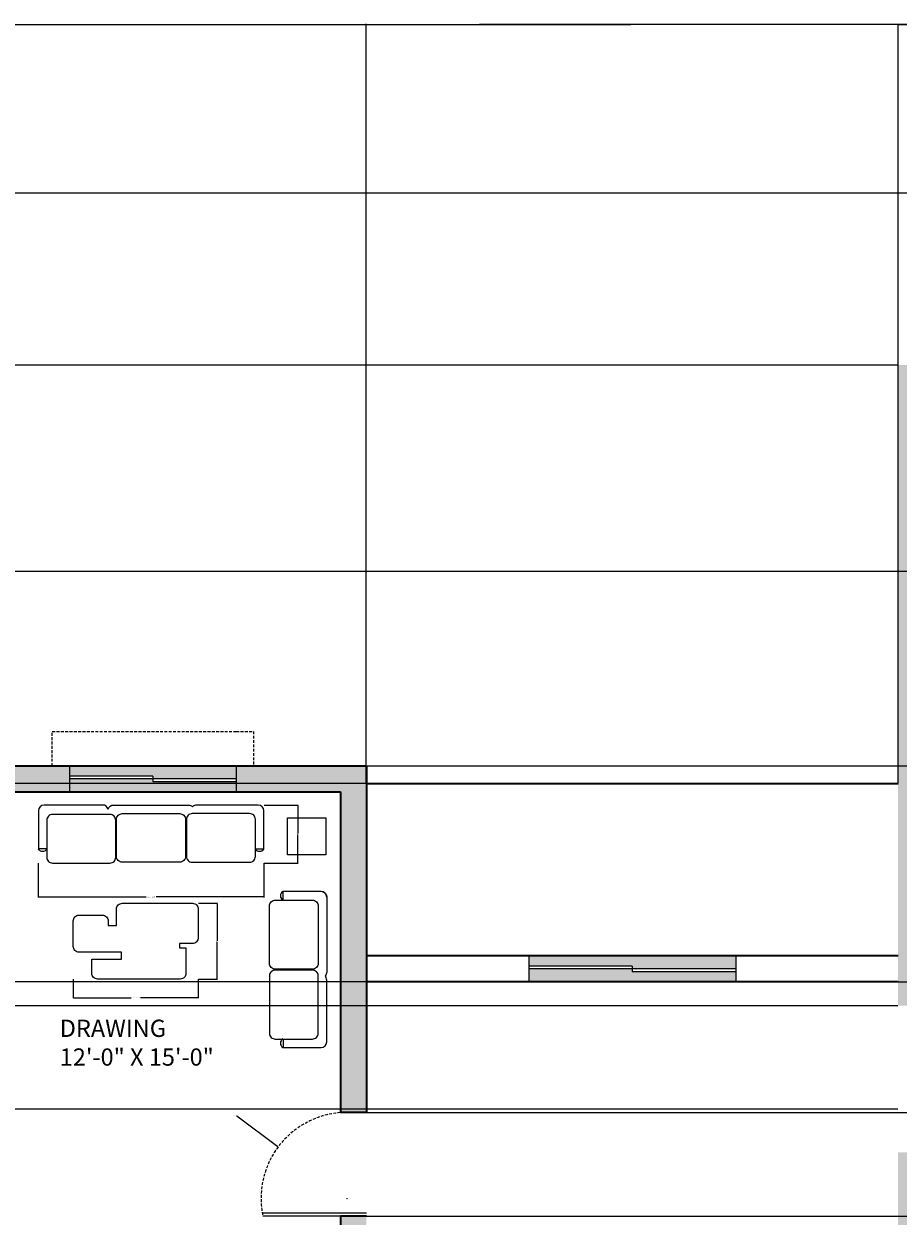
# Model space of a CAD drawing. Units: inches. Extents: x 1693 to 2974, y 2201 to 2965.
# Tile 15 of 24: x 2175 to 2479, y 2550 to 2965. Entities that reach past the tile are written whole.
import ezdxf

# ---------------------------------------------------------------- set-up
doc = ezdxf.new("R2010")
doc.units = ezdxf.units.IN
doc.header["$LTSCALE"] = 2
doc.header["$MEASUREMENT"] = 0
doc.linetypes.add('HIDDEN', pattern=[0.375, 0.25, -0.125])
for name, color, linetype, lineweight in [('A-ANNO-DIMS', 2, 'Continuous', 18), ('A-AREA-IDEN', 7, 'Continuous', 18), ('A-DOOR', 3, 'Continuous', 25), ('A-DOOR-SWNG', 3, 'HIDDEN', 13), ('A-FURN', 8, 'Continuous', 18), ('A-GLAZ', 4, 'Continuous', 18), ('A-GLAZ-OVHD', 8, 'HIDDEN', 13), ('A-WALL', 7, 'Continuous', 35)]:
    doc.layers.add(name, color=color, linetype=linetype, lineweight=lineweight)
doc.layers.add('A-GLAZ-PATT', color=141, linetype='Continuous', lineweight=13, true_color=0xadddf7)
doc.layers.add('A-WALL-PATT', color=251, linetype='Continuous', lineweight=13, true_color=0x636466)
doc.styles.get("Standard").update_dxf_attribs({"font": 'arial.ttf'})
doc.dimstyles.get("Standard").update_dxf_attribs({"dimtxt": 0.18, "dimasz": 0.18, "dimexe": 0.18, "dimexo": 0.0625, "dimgap": 0.09, "dimtad": 0, "dimtih": 1, "dimtoh": 1, "dimdec": 1, "dimzin": 0, "dimdsep": 46, "dimlunit": 3, "dimtxsty": 'Standard', "dimcen": 0.09, "dimadec": 0, "dimazin": 0, "dimtfac": 1, "dimtdec": 1, "dimtofl": 0, "dimtmove": 0, "dimatfit": 3, "dimfxl": 1, "dimtolj": 1, "dimtzin": 0, "dimarcsym": 0})

# ---------------------------------------------------------------- blocks, each defined once
blk = doc.blocks.new('SOFA-2-SEAT')
at = {"ltscale": 2}
for p, q in [((17.9, 54.27), (4.68, 54.27)), ((4.68, 51.27), (4.68, 54.27)), ((4.68, 51.27), (4.68, 51.55)), ((4.68, 27.26), (4.68, 26.96)), ((19.9, 2), (19.9, 23.43)), ((4.59, 0), (17.9, 0)), ((4.68, 3), (4.68, 0))]:
    blk.add_line(p, q, dxfattribs=at)
for points in [[(18.47, 54.18, -0.331344), (19.9, 52.27), (19.9, 26.26, -0.198912), (19.31, 24.85)], [(0, 49.27, -0.414214), (2, 51.27), (14.9, 51.27, -0.414214), (16.9, 49.27), (16.9, 29.26, -0.414214), (14.9, 27.26), (2, 27.26, -0.414214), (0, 29.26), (0, 49.27)], [(0, 4.95, 0.414214), (2, 2.95), (14.9, 2.95, 0.414214), (16.9, 4.95), (16.9, 24.96, 0.414214), (14.9, 26.96), (2, 26.96, 0.414214), (0, 24.96), (0, 4.95)]]:
    blk.add_lwpolyline(points, format="xyb", dxfattribs=at)
for centre, radius, start, end in [((5.65, 52.79), 1.86, 125.0084, 234.9916), ((17.9, 52.27), 2, 0, 90), ((5.65, 52.75), 1.86, 219.881, 234.9916), ((5.65, 25.74), 1.86, 125.0084, 139.1343), ((17.9, 23.43), 2, 0, 45), ((5.65, 1.52), 1.86, 125.0084, 234.9916), ((17.9, 2), 2, 270, 0)]:
    blk.add_arc(centre, radius, start, end, dxfattribs=at)
blk = doc.blocks.new('SOFA-3-SEAT')
at = {"ltscale": 2}
for p, q in [((0.05, 18.19), (0.05, 4.98)), ((22.37, 20.19), (2.05, 20.19)), ((76.47, 20.19), (55.04, 20.19)), ((78.47, 4.88), (78.47, 18.19)), ((3.05, 4.98), (0.05, 4.98)), ((27.21, 4.98), (26.92, 4.98)), ((51.21, 4.98), (51.52, 4.98)), ((75.47, 4.98), (78.47, 4.98))]:
    blk.add_line(p, q, dxfattribs=at)
for points in [[(24.92, 0, 0.414214), (26.92, 2), (26.92, 14.9, 0.414214), (24.92, 16.9), (4.92, 16.9, 0.414214), (2.92, 14.9), (2.92, 2, 0.414214), (4.92, 0), (24.92, 0)], [(24.29, 18.76, -0.331344), (26.21, 20.19), (52.21, 20.19, -0.198912), (53.63, 19.6)], [(29.21, 0.29, -0.414214), (27.21, 2.29), (27.21, 15.19, -0.414214), (29.21, 17.19), (49.21, 17.19, -0.414214), (51.21, 15.19), (51.21, 2.29, -0.414214), (49.21, 0.29), (29.21, 0.29)], [(73.52, 0.29, 0.414214), (75.52, 2.29), (75.52, 15.19, 0.414214), (73.52, 17.19), (53.52, 17.19, 0.414214), (51.52, 15.19), (51.52, 2.29, 0.414214), (53.52, 0.29), (73.52, 0.29)]]:
    blk.add_lwpolyline(points, format="xyb", dxfattribs=at)
for centre, radius, start, end in [((2.05, 18.19), 2, 90, 180), ((22.37, 18.19), 2, 16.6709, 90), ((55.04, 18.19), 2, 90, 135), ((76.47, 18.19), 2, 0, 90), ((1.52, 5.95), 1.86, 215.0084, 324.9916), ((25.73, 5.95), 1.86, 309.881, 324.9916), ((52.73, 5.95), 1.86, 215.0084, 229.1343), ((76.95, 5.95), 1.86, 215.0084, 324.9916)]:
    blk.add_arc(centre, radius, start, end, dxfattribs=at)
blk = doc.blocks.new('TABLE-COCKTAIL')
at = {"ltscale": 2}
blk.add_lwpolyline([(17.32, 26.34), (41.47, 26.34, -0.414214), (43.47, 24.34), (43.47, 14.36, -0.414214), (41.47, 12.36), (36.89, 12.36), (36.89, 10.89), (39.2, 10.89), (39.2, 2, -0.414214), (37.2, 0), (8.45, 0, -0.414214), (6.45, 2), (6.45, 6.97), (16.72, 6.97), (16.72, 9.34), (2, 9.34, -0.414214), (0, 11.34), (0, 20.23, -0.414214), (2, 22.23), (10.11, 22.23, -0.414214), (12.11, 20.23), (12.11, 18.68), (15.01, 18.68), (15.01, 24.34, -0.414214), (17.01, 26.34), (17.32, 26.34)], format="xyb", dxfattribs=at)
blk = doc.blocks.new('TABLE-END-SQUARE')
at = {"ltscale": 2}
blk.add_lwpolyline([(0, 12.88), (13.32, 12.88), (13.32, 0), (0, 0)], close=True, dxfattribs=at)
blk = doc.blocks.new('*D63')
at = {"layer": 'A-ANNO-DIMS', "color": 0, "lineweight": -2, "ltscale": 2, "transparency": 16777216}
for p, q in [((2180.12, 2673.01), (2180.12, 2661.12)), ((2258.59, 2673.01), (2258.59, 2661.12)), ((2180.3, 2661.3), (2217.62, 2661.3)), ((2258.41, 2661.3), (2221.09, 2661.3))]:
    blk.add_line(p, q, dxfattribs=at)
at = {"layer": 'A-ANNO-DIMS', "color": 0, "ltscale": 2, "transparency": 16777216}
for points in [[(2180.3, 2661.33), (2180.3, 2661.27), (2180.12, 2661.3)], [(2258.41, 2661.33), (2258.41, 2661.27), (2258.59, 2661.3)]]:
    blk.add_solid(points, dxfattribs=at)
at = {"layer": 'Defpoints', "color": 0, "ltscale": 2, "transparency": 16777216}
for p in [(2180.12, 2673.08), (2258.59, 2673.08), (2258.59, 2661.3)]:
    blk.add_point(p, dxfattribs=at)
at = {"layer": 'A-ANNO-DIMS', "color": 0, "ltscale": 2, "transparency": 16777216, "insert": (2219.35, 2661.3), "char_height": 0.18, "attachment_point": 5}
blk.add_mtext('\\A1;THREE-SEAT SOFA 78 TYP.', dxfattribs=at)
blk = doc.blocks.new('*D64')
at = {"layer": 'A-ANNO-DIMS', "color": 0, "lineweight": -2, "ltscale": 2, "transparency": 16777216}
for p, q in [((2258.65, 2693.26), (2270.54, 2693.26)), ((2270.36, 2693.08), (2270.36, 2683.35)), ((2270.36, 2673.26), (2270.36, 2682.99)), ((2258.65, 2673.08), (2270.54, 2673.08))]:
    blk.add_line(p, q, dxfattribs=at)
at = {"layer": 'A-ANNO-DIMS', "color": 0, "ltscale": 2, "transparency": 16777216}
for points in [[(2270.33, 2693.08), (2270.39, 2693.08), (2270.36, 2693.26)], [(2270.33, 2673.26), (2270.39, 2673.26), (2270.36, 2673.08)]]:
    blk.add_solid(points, dxfattribs=at)
at = {"layer": 'Defpoints', "color": 0, "ltscale": 2, "transparency": 16777216}
for p in [(2258.59, 2693.26), (2270.36, 2693.26), (2258.59, 2673.08)]:
    blk.add_point(p, dxfattribs=at)
at = {"layer": 'A-ANNO-DIMS', "color": 0, "ltscale": 2, "transparency": 16777216, "insert": (2270.36, 2683.17), "char_height": 0.18, "attachment_point": 5}
blk.add_mtext('\\A1;20 TYP.', dxfattribs=at)
blk = doc.blocks.new('*D69')
at = {"layer": 'A-ANNO-DIMS', "color": 0, "lineweight": -2, "ltscale": 2, "transparency": 16777216}
for p, q in [((2192.29, 2632.67), (2192.29, 2626.03)), ((2235.76, 2632.67), (2235.76, 2626.03)), ((2192.47, 2626.21), (2212.4, 2626.21)), ((2235.58, 2626.21), (2215.65, 2626.21))]:
    blk.add_line(p, q, dxfattribs=at)
at = {"layer": 'A-ANNO-DIMS', "color": 0, "ltscale": 2, "transparency": 16777216}
for points in [[(2192.47, 2626.24), (2192.47, 2626.18), (2192.29, 2626.21)], [(2235.58, 2626.24), (2235.58, 2626.18), (2235.76, 2626.21)]]:
    blk.add_solid(points, dxfattribs=at)
at = {"layer": 'Defpoints', "color": 0, "ltscale": 2, "transparency": 16777216}
for p in [(2192.29, 2632.73), (2235.76, 2632.73), (2235.76, 2626.21)]:
    blk.add_point(p, dxfattribs=at)
at = {"layer": 'A-ANNO-DIMS', "color": 0, "ltscale": 2, "transparency": 16777216, "insert": (2214.03, 2626.21), "char_height": 0.18, "attachment_point": 5}
blk.add_mtext('\\A1;COCKTAIL TABLE 43 TYP.', dxfattribs=at)
blk = doc.blocks.new('*D70')
at = {"layer": 'A-ANNO-DIMS', "color": 0, "lineweight": -2, "ltscale": 2, "transparency": 16777216}
for p, q in [((2235.82, 2659.07), (2242.46, 2659.07)), ((2242.28, 2658.89), (2242.28, 2646.08)), ((2242.28, 2632.91), (2242.28, 2645.72)), ((2235.82, 2632.73), (2242.46, 2632.73))]:
    blk.add_line(p, q, dxfattribs=at)
at = {"layer": 'A-ANNO-DIMS', "color": 0, "ltscale": 2, "transparency": 16777216}
for points in [[(2242.25, 2658.89), (2242.31, 2658.89), (2242.28, 2659.07)], [(2242.25, 2632.91), (2242.31, 2632.91), (2242.28, 2632.73)]]:
    blk.add_solid(points, dxfattribs=at)
at = {"layer": 'Defpoints', "color": 0, "ltscale": 2, "transparency": 16777216}
for p in [(2235.76, 2659.07), (2242.28, 2659.07), (2235.76, 2632.73)]:
    blk.add_point(p, dxfattribs=at)
at = {"layer": 'A-ANNO-DIMS', "color": 0, "ltscale": 2, "transparency": 16777216, "insert": (2242.28, 2645.9), "char_height": 0.18, "attachment_point": 5}
blk.add_mtext('\\A1;26 TYP.', dxfattribs=at)
blk = doc.blocks.new('*D81')
at = {"layer": 'A-ANNO-DIMS', "color": 0, "lineweight": -2, "ltscale": 2, "transparency": 16777216}
for p, q in [((1752.34, 2553.91), (1752.34, 2964.96)), ((1752.52, 2964.78), (2332.94, 2964.78)), ((2914.06, 2964.78), (2333.64, 2964.78)), ((2914.24, 2754.97), (2914.24, 2964.96))]:
    blk.add_line(p, q, dxfattribs=at)
at = {"layer": 'A-ANNO-DIMS', "color": 0, "ltscale": 2, "transparency": 16777216}
for points in [[(1752.52, 2964.81), (1752.52, 2964.75), (1752.34, 2964.78)], [(2914.06, 2964.81), (2914.06, 2964.75), (2914.24, 2964.78)]]:
    blk.add_solid(points, dxfattribs=at)
at = {"layer": 'Defpoints', "color": 0, "ltscale": 2, "transparency": 16777216}
for p in [(2914.24, 2964.78), (2914.24, 2754.9), (1752.34, 2553.84)]:
    blk.add_point(p, dxfattribs=at)
at = {"layer": 'A-ANNO-DIMS', "color": 0, "ltscale": 2, "transparency": 16777216, "insert": (2333.29, 2964.78), "char_height": 0.18, "attachment_point": 5}
blk.add_mtext('\\A1;1162', dxfattribs=at)
blk = doc.blocks.new('*D82')
at = {"layer": 'A-ANNO-DIMS', "color": 0, "lineweight": -2, "ltscale": 2, "transparency": 16777216}
for p, q in [((2615.67, 2906.08), (1693.46, 2906.08)), ((1693.64, 2905.9), (1693.64, 2582.94)), ((1693.64, 2259.62), (1693.64, 2582.58)), ((2096.17, 2259.44), (1693.46, 2259.44))]:
    blk.add_line(p, q, dxfattribs=at)
at = {"layer": 'A-ANNO-DIMS', "color": 0, "ltscale": 2, "transparency": 16777216}
for points in [[(1693.61, 2905.9), (1693.67, 2905.9), (1693.64, 2906.08)], [(1693.61, 2259.62), (1693.67, 2259.62), (1693.64, 2259.44)]]:
    blk.add_solid(points, dxfattribs=at)
at = {"layer": 'Defpoints', "color": 0, "ltscale": 2, "transparency": 16777216}
for p in [(1693.64, 2906.08), (2615.74, 2906.08), (2096.24, 2259.44)]:
    blk.add_point(p, dxfattribs=at)
at = {"layer": 'A-ANNO-DIMS', "color": 0, "ltscale": 2, "transparency": 16777216, "insert": (1693.64, 2582.76), "char_height": 0.18, "attachment_point": 5}
blk.add_mtext('\\A1;646.6', dxfattribs=at)
blk = doc.blocks.new('*D84')
at = {"layer": 'A-ANNO-DIMS', "color": 0, "lineweight": -2, "ltscale": 2, "transparency": 16777216}
for p, q in [((2294.17, 2700.82), (2294.17, 2964.96)), ((2294.35, 2964.78), (2386.25, 2964.78)), ((2479.06, 2964.78), (2387.16, 2964.78)), ((2479.24, 2700.82), (2479.24, 2964.96))]:
    blk.add_line(p, q, dxfattribs=at)
at = {"layer": 'A-ANNO-DIMS', "color": 0, "ltscale": 2, "transparency": 16777216}
for points in [[(2294.35, 2964.81), (2294.35, 2964.75), (2294.17, 2964.78)], [(2479.06, 2964.81), (2479.06, 2964.75), (2479.24, 2964.78)]]:
    blk.add_solid(points, dxfattribs=at)
at = {"layer": 'Defpoints', "color": 0, "ltscale": 2, "transparency": 16777216}
for p in [(2479.24, 2964.78), (2294.17, 2700.75), (2479.24, 2700.75)]:
    blk.add_point(p, dxfattribs=at)
at = {"layer": 'A-ANNO-DIMS', "color": 0, "ltscale": 2, "transparency": 16777216, "insert": (2386.7, 2964.78), "char_height": 0.18, "attachment_point": 5}
blk.add_mtext('\\A1;185.07', dxfattribs=at)
blk = doc.blocks.new('*D88')
at = {"layer": 'A-ANNO-DIMS', "color": 0, "lineweight": -2, "ltscale": 2, "transparency": 16777216}
for p, q in [((2479.17, 2700.75), (1693.46, 2700.75)), ((1693.64, 2700.57), (1693.64, 2666.44)), ((1693.64, 2631.93), (1693.64, 2666.07)), ((2479.17, 2631.75), (1693.46, 2631.75))]:
    blk.add_line(p, q, dxfattribs=at)
at = {"layer": 'A-ANNO-DIMS', "color": 0, "ltscale": 2, "transparency": 16777216}
for points in [[(1693.61, 2700.57), (1693.67, 2700.57), (1693.64, 2700.75)], [(1693.61, 2631.93), (1693.67, 2631.93), (1693.64, 2631.75)]]:
    blk.add_solid(points, dxfattribs=at)
at = {"layer": 'Defpoints', "color": 0, "ltscale": 2, "transparency": 16777216}
for p in [(1693.64, 2700.75), (2479.24, 2700.75), (2479.24, 2631.75)]:
    blk.add_point(p, dxfattribs=at)
at = {"layer": 'A-ANNO-DIMS', "color": 0, "ltscale": 2, "transparency": 16777216, "insert": (1693.64, 2666.25), "char_height": 0.18, "attachment_point": 5}
blk.add_mtext('\\A1;69', dxfattribs=at)
blk = doc.blocks.new('*D90')
at = {"layer": 'A-ANNO-DIMS', "color": 0, "lineweight": -2, "ltscale": 2, "transparency": 16777216}
for p, q in [((2145.8, 2774.54), (2973.12, 2774.54)), ((2972.94, 2774.36), (2972.94, 2740.87)), ((2972.94, 2707.02), (2972.94, 2740.51)), ((2294.3, 2706.84), (2973.12, 2706.84))]:
    blk.add_line(p, q, dxfattribs=at)
at = {"layer": 'A-ANNO-DIMS', "color": 0, "ltscale": 2, "transparency": 16777216}
for points in [[(2972.91, 2774.36), (2972.97, 2774.36), (2972.94, 2774.54)], [(2972.91, 2707.02), (2972.97, 2707.02), (2972.94, 2706.84)]]:
    blk.add_solid(points, dxfattribs=at)
at = {"layer": 'Defpoints', "color": 0, "ltscale": 2, "transparency": 16777216}
for p in [(2145.74, 2774.54), (2294.24, 2706.84), (2972.94, 2706.84)]:
    blk.add_point(p, dxfattribs=at)
at = {"layer": 'A-ANNO-DIMS', "color": 0, "ltscale": 2, "transparency": 16777216, "insert": (2972.94, 2740.69), "char_height": 0.18, "attachment_point": 5}
blk.add_mtext('\\A1;67.7', dxfattribs=at)
blk = doc.blocks.new('*D91')
at = {"layer": 'A-ANNO-DIMS', "color": 0, "lineweight": -2, "ltscale": 2, "transparency": 16777216}
for p, q in [((2615.67, 2906.08), (1693.46, 2906.08)), ((1693.64, 2905.9), (1693.64, 2876.35)), ((1693.64, 2846.43), (1693.64, 2875.98)), ((2479.17, 2846.25), (1693.46, 2846.25))]:
    blk.add_line(p, q, dxfattribs=at)
at = {"layer": 'A-ANNO-DIMS', "color": 0, "ltscale": 2, "transparency": 16777216}
for points in [[(1693.61, 2905.9), (1693.67, 2905.9), (1693.64, 2906.08)], [(1693.61, 2846.43), (1693.67, 2846.43), (1693.64, 2846.25)]]:
    blk.add_solid(points, dxfattribs=at)
at = {"layer": 'Defpoints', "color": 0, "ltscale": 2, "transparency": 16777216}
for p in [(2615.74, 2906.08), (1693.64, 2846.25), (2479.24, 2846.25)]:
    blk.add_point(p, dxfattribs=at)
at = {"layer": 'A-ANNO-DIMS', "color": 0, "ltscale": 2, "transparency": 16777216, "insert": (1693.64, 2876.17), "char_height": 0.18, "attachment_point": 5}
blk.add_mtext('\\A1;59.82', dxfattribs=at)
blk = doc.blocks.new('*D96')
at = {"layer": 'A-ANNO-DIMS', "color": 0, "lineweight": -2, "ltscale": 2, "transparency": 16777216}
for p, q in [((2294.3, 2586.26), (2973.12, 2586.26)), ((2972.94, 2586.08), (2972.94, 2568.45)), ((2972.94, 2550.44), (2972.94, 2568.08)), ((2294.3, 2550.26), (2973.12, 2550.26))]:
    blk.add_line(p, q, dxfattribs=at)
at = {"layer": 'A-ANNO-DIMS', "color": 0, "ltscale": 2, "transparency": 16777216}
for points in [[(2972.91, 2586.08), (2972.97, 2586.08), (2972.94, 2586.26)], [(2972.91, 2550.44), (2972.97, 2550.44), (2972.94, 2550.26)]]:
    blk.add_solid(points, dxfattribs=at)
at = {"layer": 'Defpoints', "color": 0, "ltscale": 2, "transparency": 16777216}
for p in [(2294.24, 2586.26), (2972.94, 2586.26), (2294.24, 2550.26)]:
    blk.add_point(p, dxfattribs=at)
at = {"layer": 'A-ANNO-DIMS', "color": 0, "ltscale": 2, "transparency": 16777216, "insert": (2972.94, 2568.26), "char_height": 0.18, "attachment_point": 5}
blk.add_mtext('\\A1;36', dxfattribs=at)
blk = doc.blocks.new('*D97')
at = {"layer": 'A-ANNO-DIMS', "color": 0, "lineweight": -2, "ltscale": 2, "transparency": 16777216}
for p, q in [((2294.3, 2631.75), (2973.12, 2631.75)), ((2972.94, 2631.57), (2972.94, 2609.19)), ((2972.94, 2586.44), (2972.94, 2608.83)), ((2294.3, 2586.26), (2973.12, 2586.26))]:
    blk.add_line(p, q, dxfattribs=at)
at = {"layer": 'A-ANNO-DIMS', "color": 0, "ltscale": 2, "transparency": 16777216}
for points in [[(2972.91, 2631.57), (2972.97, 2631.57), (2972.94, 2631.75)], [(2972.91, 2586.44), (2972.97, 2586.44), (2972.94, 2586.26)]]:
    blk.add_solid(points, dxfattribs=at)
at = {"layer": 'Defpoints', "color": 0, "ltscale": 2, "transparency": 16777216}
for p in [(2294.24, 2631.75), (2972.94, 2631.75), (2294.24, 2586.26)]:
    blk.add_point(p, dxfattribs=at)
at = {"layer": 'A-ANNO-DIMS', "color": 0, "ltscale": 2, "transparency": 16777216, "insert": (2972.94, 2609.01), "char_height": 0.18, "attachment_point": 5}
blk.add_mtext('\\A1;45.49', dxfattribs=at)
blk = doc.blocks.new('*D98')
at = {"layer": 'A-ANNO-DIMS', "color": 0, "lineweight": -2, "ltscale": 2, "transparency": 16777216}
for p, q in [((2479.17, 2623.46), (1693.46, 2623.46)), ((1693.64, 2623.28), (1693.64, 2605.64)), ((1693.64, 2587.64), (1693.64, 2605.28)), ((2479.17, 2587.46), (1693.46, 2587.46))]:
    blk.add_line(p, q, dxfattribs=at)
at = {"layer": 'A-ANNO-DIMS', "color": 0, "ltscale": 2, "transparency": 16777216}
for points in [[(1693.61, 2623.28), (1693.67, 2623.28), (1693.64, 2623.46)], [(1693.61, 2587.64), (1693.67, 2587.64), (1693.64, 2587.46)]]:
    blk.add_solid(points, dxfattribs=at)
at = {"layer": 'Defpoints', "color": 0, "ltscale": 2, "transparency": 16777216}
for p in [(1693.64, 2623.46), (2479.24, 2623.46), (2479.24, 2587.46)]:
    blk.add_point(p, dxfattribs=at)
at = {"layer": 'A-ANNO-DIMS', "color": 0, "ltscale": 2, "transparency": 16777216, "insert": (1693.64, 2605.46), "char_height": 0.18, "attachment_point": 5}
blk.add_mtext('\\A1;36', dxfattribs=at)
blk = doc.blocks.new('*D99')
at = {"layer": 'A-ANNO-DIMS', "color": 0, "lineweight": -2, "ltscale": 2, "transparency": 16777216}
for p, q in [((2479.17, 2631.75), (1693.46, 2631.75)), ((1693.64, 2631.57), (1693.64, 2627.79)), ((1693.64, 2623.64), (1693.64, 2627.43)), ((2479.17, 2623.46), (1693.46, 2623.46))]:
    blk.add_line(p, q, dxfattribs=at)
at = {"layer": 'A-ANNO-DIMS', "color": 0, "ltscale": 2, "transparency": 16777216}
for points in [[(1693.61, 2631.57), (1693.67, 2631.57), (1693.64, 2631.75)], [(1693.61, 2623.64), (1693.67, 2623.64), (1693.64, 2623.46)]]:
    blk.add_solid(points, dxfattribs=at)
at = {"layer": 'Defpoints', "color": 0, "ltscale": 2, "transparency": 16777216}
for p in [(1693.64, 2631.75), (2479.24, 2631.75), (2479.24, 2623.46)]:
    blk.add_point(p, dxfattribs=at)
at = {"layer": 'A-ANNO-DIMS', "color": 0, "ltscale": 2, "transparency": 16777216, "insert": (1693.64, 2627.61), "char_height": 0.18, "attachment_point": 5}
blk.add_mtext('\\A1;8.295', dxfattribs=at)
blk = doc.blocks.new('*D101')
at = {"layer": 'A-ANNO-DIMS', "color": 0, "lineweight": -2, "ltscale": 2, "transparency": 16777216}
for p, q in [((2479.24, 2846.32), (2479.24, 2964.96)), ((2479.42, 2964.78), (2547.1, 2964.78)), ((2615.56, 2964.78), (2547.87, 2964.78)), ((2615.74, 2846.32), (2615.74, 2964.96))]:
    blk.add_line(p, q, dxfattribs=at)
at = {"layer": 'A-ANNO-DIMS', "color": 0, "ltscale": 2, "transparency": 16777216}
for points in [[(2479.42, 2964.81), (2479.42, 2964.75), (2479.24, 2964.78)], [(2615.56, 2964.81), (2615.56, 2964.75), (2615.74, 2964.78)]]:
    blk.add_solid(points, dxfattribs=at)
at = {"layer": 'Defpoints', "color": 0, "ltscale": 2, "transparency": 16777216}
for p in [(2615.74, 2964.78), (2479.24, 2846.25), (2615.74, 2846.25)]:
    blk.add_point(p, dxfattribs=at)
at = {"layer": 'A-ANNO-DIMS', "color": 0, "ltscale": 2, "transparency": 16777216, "insert": (2547.49, 2964.78), "char_height": 0.18, "attachment_point": 5}
blk.add_mtext('\\A1;136.5', dxfattribs=at)
blk = doc.blocks.new('*D121')
at = {"layer": 'A-ANNO-DIMS', "color": 0, "lineweight": -2, "ltscale": 2, "transparency": 16777216}
for p, q in [((2249.04, 2585.16), (2249.22, 2585.16)), ((2249.22, 2585.16), (2263.44, 2574.49)), ((2287.43, 2556.43), (2287.61, 2556.43)), ((2287.52, 2556.34), (2287.52, 2556.52))]:
    blk.add_line(p, q, dxfattribs=at)
at = {"layer": 'A-ANNO-DIMS', "color": 0, "ltscale": 2, "transparency": 16777216}
blk.add_solid([(2263.45, 2574.51), (2263.42, 2574.47), (2263.58, 2574.38)], dxfattribs=at)
at = {"layer": 'Defpoints', "color": 0, "ltscale": 2, "transparency": 16777216}
for p in [(2263.58, 2574.38), (2287.52, 2556.43)]:
    blk.add_point(p, dxfattribs=at)
at = {"layer": 'A-ANNO-DIMS', "color": 0, "ltscale": 2, "transparency": 16777216, "insert": (2248.49, 2585.16), "char_height": 0.18, "attachment_point": 5}
blk.add_mtext('\\A1;R29.925', dxfattribs=at)

msp = doc.modelspace()

# ---------------------------------------------------------------- hatches: boundary and pattern name
at = {"layer": 'A-GLAZ-PATT', "ltscale": 2}
h = msp.add_hatch(color=256, dxfattribs=at)
h.dxf.hatch_style = 1
h.paths.add_polyline_path([(2656.9702, 2338.2547), (2632.9702, 2338.2547), (2632.9702, 2339.2547), (2608.9702, 2339.2547), (2608.9702, 2334.7547), (2656.9702, 2334.7547)])
h.paths.add_polyline_path([(2656.9702, 2343.7547), (2608.9702, 2343.7547), (2608.9702, 2340.2547), (2632.9702, 2340.2547), (2632.9702, 2339.2547), (2656.9702, 2339.2547)])
h.paths.add_polyline_path([(2775.7544, 2338.2547), (2751.7544, 2338.2547), (2751.7544, 2334.7547), (2775.7544, 2334.7547)])
h.paths.add_polyline_path([(2775.7544, 2343.7547), (2751.7544, 2343.7547), (2751.7544, 2340.2547), (2775.7544, 2340.2547)])
h.paths.add_polyline_path([(2897.7363, 2568.7999), (2893.2363, 2568.7999), (2893.2363, 2520.7999), (2896.7363, 2520.7999), (2896.7363, 2544.7999), (2897.7363, 2544.7999)])
h.paths.add_polyline_path([(2902.2363, 2568.7999), (2898.7363, 2568.7999), (2898.7363, 2544.7999), (2897.7363, 2544.7999), (2897.7363, 2520.7999), (2902.2363, 2520.7999)])
h.paths.add_polyline_path([(2902.2363, 2637.7547), (2898.7363, 2637.7547), (2898.7363, 2613.7547), (2902.2363, 2613.7547)])
h.paths.add_polyline_path([(2896.7363, 2637.7547), (2893.2363, 2637.7547), (2893.2363, 2613.7547), (2896.7363, 2613.7547)])
h.paths.add_polyline_path([(2902.2363, 2748.903), (2899.0477, 2748.903), (2899.0477, 2724.903), (2898.0477, 2724.903), (2898.0477, 2700.903), (2902.2363, 2700.903)])
h.paths.add_polyline_path([(2898.0477, 2748.903), (2893.2363, 2748.903), (2893.2363, 2700.903), (2897.0477, 2700.903), (2897.0477, 2724.903), (2898.0477, 2724.903)])
h.paths.add_polyline_path([(2851.2363, 2846.2547), (2803.2363, 2846.2547), (2803.2363, 2842.7547), (2827.2363, 2842.7547), (2827.2363, 2841.7547), (2851.2363, 2841.7547)])
h.paths.add_polyline_path([(2851.2363, 2840.7547), (2827.2363, 2840.7547), (2827.2363, 2841.7547), (2803.2363, 2841.7547), (2803.2363, 2837.2547), (2851.2363, 2837.2547)])
h.paths.add_polyline_path([(2578.2363, 2846.2547), (2530.2363, 2846.2547), (2530.2363, 2842.7547), (2554.2363, 2842.7547), (2554.2363, 2841.7547), (2578.2363, 2841.7547)])
h.paths.add_polyline_path([(2578.2363, 2840.7547), (2554.2363, 2840.7547), (2554.2363, 2841.7547), (2530.2363, 2841.7547), (2530.2363, 2837.2547), (2578.2363, 2837.2547)])
h.paths.add_polyline_path([(2732.7363, 2812.7547), (2705.1363, 2812.7547), (2705.1363, 2811.7547), (2676.3363, 2811.7547), (2676.3363, 2812.7547), (2648.7363, 2812.7547), (2648.7363, 2808.2547), (2732.7363, 2808.2547)])
h.paths.add_polyline_path([(2732.7363, 2817.2547), (2648.7363, 2817.2547), (2648.7363, 2813.7547), (2676.3363, 2813.7547), (2676.3363, 2812.7547), (2705.1363, 2812.7547), (2705.1363, 2813.7547), (2732.7363, 2813.7547)])
h.paths.add_polyline_path([(2488.2363, 2695.8203), (2484.7878, 2695.8203), (2484.7878, 2671.8203), (2488.2363, 2671.8203)])
h.paths.add_polyline_path([(2482.7878, 2695.8203), (2479.2363, 2695.8203), (2479.2363, 2671.8203), (2482.7878, 2671.8203)])
h.paths.add_polyline_path([(2488.2363, 2572.4371), (2484.7363, 2572.4371), (2484.7363, 2541.4371), (2483.7363, 2541.4371), (2483.7363, 2512.4371), (2488.2363, 2512.4371)])
h.paths.add_polyline_path([(2482.7363, 2541.4371), (2483.7363, 2541.4371), (2483.7363, 2572.4371), (2479.2363, 2572.4371), (2479.2363, 2512.4371), (2482.7363, 2512.4371)])
h.paths.add_polyline_path([(2248.9863, 2706.8449), (2190.9863, 2706.8449), (2190.9863, 2703.3449), (2219.9863, 2703.3449), (2219.9863, 2702.3449), (2248.9863, 2702.3449)])
h.paths.add_polyline_path([(2248.9863, 2701.3449), (2219.9863, 2701.3449), (2219.9863, 2702.3449), (2190.9863, 2702.3449), (2190.9863, 2697.8449), (2248.9863, 2697.8449)])
h.paths.add_polyline_path([(2151.9207, 2293.3449), (2127.9207, 2293.3449), (2127.9207, 2289.8449), (2151.9207, 2289.8449)])
h.paths.add_polyline_path([(2151.9207, 2298.8449), (2127.9207, 2298.8449), (2127.9207, 2295.3449), (2151.9207, 2295.3449)])
h.paths.add_polyline_path([(2084.023, 2293.3449), (2066.023, 2293.3449), (2066.023, 2294.3449), (2048.023, 2294.3449), (2048.023, 2289.8449), (2084.023, 2289.8449)])
h.paths.add_polyline_path([(2084.023, 2298.8449), (2048.023, 2298.8449), (2048.023, 2295.3449), (2066.023, 2295.3449), (2066.023, 2294.3449), (2084.023, 2294.3449)])
h.paths.add_polyline_path([(1966.0781, 2293.3449), (1948.0781, 2293.3449), (1948.0781, 2294.3449), (1930.0781, 2294.3449), (1930.0781, 2289.8449), (1966.0781, 2289.8449)])
h.paths.add_polyline_path([(1966.0781, 2298.8449), (1930.0781, 2298.8449), (1930.0781, 2295.3449), (1948.0781, 2295.3449), (1948.0781, 2294.3449), (1966.0781, 2294.3449)])
h.paths.add_polyline_path([(1787.2363, 2403.1922), (1782.7363, 2403.1922), (1782.7363, 2355.1922), (1786.2363, 2355.1922), (1786.2363, 2379.1922), (1787.2363, 2379.1922)])
h.paths.add_polyline_path([(1791.7363, 2403.1922), (1788.2363, 2403.1922), (1788.2363, 2379.1922), (1787.2363, 2379.1922), (1787.2363, 2355.1922), (1791.7363, 2355.1922)])
h.paths.add_polyline_path([(1786.2363, 2477.5455), (1782.7363, 2477.5455), (1782.7363, 2453.5455), (1786.2363, 2453.5455)])
h.paths.add_polyline_path([(1791.7363, 2477.5455), (1788.2363, 2477.5455), (1788.2363, 2453.5455), (1791.7363, 2453.5455)])
h.paths.add_polyline_path([(1786.2363, 2621.6433), (1782.7363, 2621.6433), (1782.7363, 2585.6433), (1786.2363, 2585.6433)])
h.paths.add_polyline_path([(1791.7363, 2621.6433), (1788.2363, 2621.6433), (1788.2363, 2585.6433), (1791.7363, 2585.6433)])
h.paths.add_polyline_path([(1908.1286, 2706.8449), (1860.1286, 2706.8449), (1860.1286, 2703.3449), (1884.1286, 2703.3449), (1884.1286, 2702.3449), (1908.1286, 2702.3449)])
h.paths.add_polyline_path([(1908.1286, 2701.3449), (1884.1286, 2701.3449), (1884.1286, 2702.3449), (1860.1286, 2702.3449), (1860.1286, 2697.8449), (1908.1286, 2697.8449)])
h.paths.add_polyline_path([(1973.9863, 2706.8449), (1949.9863, 2706.8449), (1949.9863, 2703.3449), (1973.9863, 2703.3449)])
h.paths.add_polyline_path([(1973.9863, 2701.3449), (1949.9863, 2701.3449), (1949.9863, 2697.8449), (1973.9863, 2697.8449)])
h.paths.add_polyline_path([(2112.7363, 2690.3449), (2028.7363, 2690.3449), (2028.7363, 2686.8449), (2056.3363, 2686.8449), (2056.3363, 2685.8449), (2085.1363, 2685.8449), (2085.1363, 2686.8449), (2112.7363, 2686.8449)])
h.paths.add_polyline_path([(2112.7363, 2685.8449), (2085.1363, 2685.8449), (2085.1363, 2684.8449), (2056.3363, 2684.8449), (2056.3363, 2685.8449), (2028.7363, 2685.8449), (2028.7363, 2681.3449), (2112.7363, 2681.3449)])
h.paths.add_polyline_path([(2422.7363, 2640.7547), (2350.7363, 2640.7547), (2350.7363, 2637.2547), (2386.7363, 2637.2547), (2386.7363, 2636.2547), (2422.7363, 2636.2547)])
h.paths.add_polyline_path([(2422.7363, 2635.2547), (2386.7363, 2635.2547), (2386.7363, 2636.2547), (2350.7363, 2636.2547), (2350.7363, 2631.7547), (2422.7363, 2631.7547)])
at = {"layer": 'A-WALL-PATT', "ltscale": 2}
h = msp.add_hatch(color=256, dxfattribs=at)
h.dxf.hatch_style = 1
h.paths.add_polyline_path([(1928.2363, 2733.2161), (1930.9384, 2733.2161), (1930.9384, 2737.2161), (1923.7363, 2737.2161), (1923.7363, 2706.8449), (1908.1286, 2706.8449), (1908.1286, 2697.8449), (1923.7363, 2697.8449), (1923.7363, 2692.8449), (1928.2363, 2692.8449), (1928.2363, 2697.8449), (1949.9863, 2697.8449), (1949.9863, 2706.8449), (1928.2363, 2706.8449)])
h.paths.add_polyline_path([(2004.7363, 2737.2161), (1995.7363, 2737.2161), (1995.7363, 2706.8449), (1985.6374, 2706.8449), (1973.9863, 2706.8449), (1973.9863, 2697.8449), (2000.2363, 2697.8449), (2000.2363, 2686.5348), (2000.3613, 2686.5348), (2000.3613, 2667.0432), (2000.2363, 2601.8449), (1928.2363, 2601.8449), (1928.2363, 2662.8449), (1923.7363, 2662.8449), (1923.7363, 2595.3449), (1928.2363, 2595.3449), (1928.2363, 2597.3449), (2004.7363, 2597.3449), (2004.7363, 2681.3449), (2012.7814, 2681.3449), (2028.7363, 2681.3449), (2028.7363, 2690.3449), (2004.7363, 2690.3449)])
h.paths.add_polyline_path([(2190.9863, 2706.8449), (2184.9863, 2706.8449), (2145.7363, 2706.8449), (2145.7363, 2765.3449), (2145.7363, 2774.5394), (2136.7363, 2774.5394), (2136.7363, 2756.3449), (2136.7363, 2690.3449), (2112.7363, 2690.3449), (2112.7363, 2681.3449), (2136.7363, 2681.3449), (2136.7363, 2597.3449), (2141.2363, 2597.3449), (2141.2363, 2697.8449), (2190.9863, 2697.8449)])
h.paths.add_polyline_path([(1860.1286, 2706.8449), (1782.7363, 2706.8449), (1782.7363, 2621.6433), (1791.7363, 2621.6433), (1791.7363, 2697.8449), (1860.1286, 2697.8449)])
h.paths.add_polyline_path([(1791.7363, 2585.6433), (1782.7363, 2585.6433), (1782.7363, 2562.8449), (1782.7363, 2553.8449), (1752.3363, 2553.8449), (1752.3363, 2544.2586), (1756.3363, 2544.2586), (1756.3363, 2549.3449), (1782.7363, 2549.3449), (1782.7363, 2489.2404), (1782.7363, 2477.5455), (1791.7363, 2477.5455), (1791.7363, 2493.5991), (1791.6113, 2493.5991), (1791.6113, 2513.0907), (1791.6824, 2533.7198, -0.94742783), (1791.7363, 2534.7168), (1791.7363, 2549.3449), (1863.7363, 2549.3449), (1863.7363, 2513.3449), (1866.7363, 2513.3449), (1866.7363, 2549.3449), (1924.7363, 2549.3449), (1924.7363, 2447.3449), (1924.7363, 2442.8449), (1933.7363, 2442.8449), (1933.7363, 2447.3449), (1928.2363, 2447.3449), (1928.2363, 2559.3449), (1923.7363, 2559.3449), (1923.7363, 2553.8449), (1791.7363, 2553.8449), (1791.7363, 2562.8449)])
h.paths.add_polyline_path([(1791.7363, 2442.8449), (1866.7363, 2442.8449), (1866.7363, 2447.3449), (1866.7363, 2483.3449), (1863.7363, 2483.3449), (1863.7363, 2447.3449), (1791.7363, 2447.3449), (1791.7363, 2453.5455), (1782.7363, 2453.5455), (1782.7363, 2447.3449), (1756.3363, 2447.3449), (1756.3363, 2455.7126), (1752.3363, 2455.7126), (1752.3363, 2442.8449), (1782.7363, 2442.8449), (1782.7363, 2403.1922), (1791.7363, 2403.1922)])
h.paths.add_polyline_path([(1930.0781, 2298.8449), (1791.7363, 2298.8449), (1791.7363, 2355.1922), (1782.7363, 2355.1922), (1782.7363, 2289.8449), (1930.0781, 2289.8449)])
h.paths.add_polyline_path([(2624.7363, 2883.2547), (2624.7363, 2902.6165), (2624.7363, 2906.0761), (2615.7363, 2906.0761), (2615.7363, 2892.2547), (2615.7363, 2846.2547), (2578.2363, 2846.2547), (2578.2363, 2837.2547), (2620.2363, 2837.2547), (2620.2363, 2743.2547), (2624.7363, 2743.2547), (2624.7363, 2808.2547), (2648.7363, 2808.2547), (2648.7363, 2817.2547), (2624.7363, 2817.2547)])
h.paths.add_polyline_path([(2530.2363, 2846.2547), (2479.2363, 2846.2547), (2479.2363, 2695.8203), (2488.2363, 2695.8203), (2488.2363, 2700.7547), (2567.2363, 2700.7547), (2567.2363, 2705.2547), (2488.2363, 2705.2547), (2488.2363, 2837.2547), (2530.2363, 2837.2547)])
h.paths.add_polyline_path([(2488.2363, 2487.7547), (2630.2363, 2487.7547, -0.00990191), (2630.2363, 2489.0322), (2630.2363, 2492.2547), (2488.2363, 2492.2547), (2488.2363, 2512.4371), (2479.2363, 2512.4371), (2479.2363, 2334.7547), (2608.9702, 2334.7547), (2608.9702, 2343.7547), (2488.2363, 2343.7547)])
h.paths.add_polyline_path([(2751.7544, 2343.7547), (2672.7363, 2343.7547), (2672.7363, 2409.7547), (2674.7363, 2409.7547), (2674.7363, 2413.7547), (2672.7363, 2413.7547), (2672.7363, 2487.7547), (2732.7363, 2487.7547), (2732.7363, 2413.7547), (2704.7363, 2413.7547), (2704.7363, 2409.7547), (2784.7363, 2409.7547), (2784.7363, 2343.7547), (2775.7544, 2343.7547), (2775.7544, 2334.7547), (2902.2363, 2334.7547), (2902.2363, 2520.7999), (2893.2363, 2520.7999), (2893.2363, 2413.7547), (2856.0145, 2413.7547), (2856.0145, 2409.7547), (2893.2363, 2409.7547), (2893.2363, 2343.7547), (2789.2363, 2343.7547), (2789.2363, 2409.7547), (2819.2363, 2409.7547), (2826.0145, 2409.7547), (2826.0145, 2413.7547), (2789.2363, 2413.7547), (2789.2363, 2492.2547), (2784.7363, 2492.2547), (2784.7363, 2413.7547), (2736.7363, 2413.7547), (2736.7363, 2492.2547), (2672.7363, 2492.2547), (2666.2363, 2492.2547), (2666.2363, 2487.7547), (2668.2363, 2487.7547), (2668.2363, 2343.7547), (2656.9702, 2343.7547), (2656.9702, 2334.7547), (2662.9702, 2334.7547), (2751.7544, 2334.7547)])
h.paths.add_polyline_path([(2902.2363, 2613.7547), (2893.2363, 2613.7547), (2893.2363, 2589.7547), (2785.2363, 2589.7547), (2785.2363, 2661.7547), (2790.2363, 2661.7547), (2790.2363, 2665.2547), (2761.2363, 2665.2547), (2761.2363, 2667.2547), (2756.7363, 2667.2547), (2756.7363, 2661.7547), (2781.2363, 2661.7547), (2781.2363, 2585.7547), (2893.2363, 2585.7547), (2893.2363, 2568.7999), (2902.2363, 2568.7999)])
h.paths.add_polyline_path([(2488.2363, 2671.8203), (2479.2363, 2671.8203), (2479.2363, 2645.2547), (2479.2363, 2623.4598), (2488.2363, 2623.4598), (2488.2363, 2636.2547), (2624.7363, 2636.2547), (2624.7363, 2640.7547), (2603.7363, 2640.7547), (2603.7363, 2700.7547), (2624.7363, 2700.7547), (2624.7363, 2707.2547), (2620.2363, 2707.2547), (2620.2363, 2705.2547), (2597.2363, 2705.2547), (2597.2363, 2700.7547), (2599.2363, 2700.7547), (2599.2363, 2640.7547), (2488.2363, 2640.7547)])
h.paths.add_polyline_path([(2761.2363, 2837.2547), (2803.2363, 2837.2547), (2803.2363, 2846.2547), (2797.2363, 2846.2547), (2765.7363, 2846.2547), (2756.7363, 2846.2547), (2756.7363, 2817.2547), (2732.7363, 2817.2547), (2732.7363, 2808.2547), (2756.7363, 2808.2547), (2756.7363, 2703.2547), (2761.2363, 2703.2547)])
h.paths.add_polyline_path([(2739.7489, 2433.1234), (2786.9181, 2433.1234), (2786.9181, 2455.5122), (2739.7489, 2455.5122)], flags=25)
h = msp.add_hatch(color=256, dxfattribs=at)
h.dxf.hatch_style = 1
h.paths.add_polyline_path([(2294.2363, 2706.8449), (2248.9863, 2706.8449), (2248.9863, 2697.8449), (2285.2363, 2697.8449), (2285.2363, 2586.2648), (2294.2363, 2586.2648)])
h.paths.add_polyline_path([(2294.2363, 2550.2648), (2285.2363, 2550.2648), (2285.2363, 2517.8449), (2141.2363, 2517.8449), (2141.2363, 2513.8449), (2285.2363, 2513.8449), (2285.2363, 2369.8449), (2253.0704, 2369.8449), (2253.0704, 2366.8449), (2285.2363, 2366.8449), (2285.2363, 2298.8449), (2165.2363, 2298.8449), (2165.2363, 2366.8449), (2165.2363, 2369.8449), (2165.2363, 2447.3449), (2160.7363, 2447.3449), (2160.7363, 2403.3449), (2100.7363, 2403.3449), (2100.7363, 2447.3449), (2094.2363, 2447.3449), (2094.2363, 2442.8449), (2096.2363, 2442.8449), (2096.2363, 2362.1344), (2100.7363, 2362.1344), (2100.7363, 2400.8449), (2160.7363, 2400.8449), (2160.7363, 2298.8449), (2151.9207, 2298.8449), (2151.9207, 2289.8449), (2184.7363, 2289.8449), (2184.7363, 2276.6449), (2189.2363, 2276.6449), (2189.2363, 2289.8449), (2294.2363, 2289.8449)])
h.paths.add_polyline_path([(2048.023, 2298.8449), (1976.2363, 2298.8449), (1976.2363, 2442.8449), (2058.2363, 2442.8449, -0.00822734), (2058.2363, 2443.9061), (2058.2363, 2447.3449), (2004.7363, 2447.3449), (1969.7363, 2447.3449), (1969.7363, 2442.8449), (1971.7363, 2442.8449), (1971.7363, 2298.8449), (1966.0781, 2298.8449), (1966.0781, 2289.8449), (2048.023, 2289.8449)])
h.paths.add_polyline_path([(2127.9207, 2298.8449), (2100.7363, 2298.8449), (2100.7363, 2332.1344), (2096.2363, 2332.1344), (2096.2363, 2298.8449), (2084.023, 2298.8449), (2084.023, 2289.8449), (2096.2363, 2289.8449), (2096.2363, 2259.4449), (2114.3201, 2259.4449), (2114.3201, 2263.4449), (2100.7363, 2263.4449), (2100.7363, 2289.8449), (2127.9207, 2289.8449)])

# ---------------------------------------------------------------- linework, layer by layer
at = {"layer": 'A-DOOR', "ltscale": 2}
for p, q in [((2294.2363, 2551.2648), (2258.2363, 2551.2648)), ((2294.2363, 2550.2648), (2258.2363, 2550.2648))]:
    msp.add_line(p, q, dxfattribs=at)
at = {"layer": 'A-DOOR-SWNG', "ltscale": 2}
msp.add_arc((2287.5204, 2556.4267), 29.9253, 94.37736, 191.882845, dxfattribs=at)
at = {"layer": 'A-GLAZ', "ltscale": 2}
for p, q in [((2190.9863, 2706.8449), (2190.9863, 2697.8449)), ((2248.9863, 2706.8449), (2248.9863, 2697.8449)), ((2219.9863, 2703.3449), (2190.9863, 2703.3449)), ((2248.9863, 2702.3449), (2190.9863, 2702.3449)), ((2219.9863, 2703.3449), (2219.9863, 2701.3449)), ((2248.9863, 2701.3449), (2219.9863, 2701.3449)), ((2350.7363, 2640.7547), (2350.7363, 2631.7547)), ((2422.7363, 2640.7547), (2422.7363, 2631.7547)), ((2386.7363, 2637.2547), (2350.7363, 2637.2547)), ((2422.7363, 2636.2547), (2350.7363, 2636.2547)), ((2386.7363, 2637.2547), (2386.7363, 2635.2547)), ((2422.7363, 2635.2547), (2386.7363, 2635.2547))]:
    msp.add_line(p, q, dxfattribs=at)
at = {"layer": 'A-GLAZ-OVHD', "ltscale": 2}
for p, q in [((2184.9863, 2706.8449), (2184.9863, 2718.8449)), ((2184.9863, 2718.8449), (2248.9863, 2718.8449)), ((2248.9863, 2718.8449), (2254.9863, 2718.8449)), ((2254.9863, 2718.8449), (2254.9863, 2706.8449)), ((2190.9863, 2706.8449), (2184.9863, 2706.8449))]:
    msp.add_line(p, q, dxfattribs=at)
at = {"layer": 'A-WALL'}
for p, q in [((2145.7363, 2706.8449), (2294.2363, 2706.8449)), ((2294.2363, 2706.8449), (2294.2363, 2586.2648)), ((2141.2363, 2697.8449), (2285.2363, 2697.8449)), ((2285.2363, 2697.8449), (2285.2363, 2586.2648)), ((2285.2363, 2550.2648), (2285.2363, 2517.8449))]:
    msp.add_line(p, q, dxfattribs=at)
at = {"layer": 'A-WALL', "ltscale": 2}
for p, q in [((2294.166, 2700.7547), (2479.2363, 2700.7547)), ((2479.2363, 2640.7547), (2294.2363, 2640.7547)), ((2479.2363, 2631.7547), (2294.2363, 2631.7547)), ((2294.2363, 2586.2648), (2285.2363, 2586.2648)), ((2294.2363, 2550.2648), (2285.2363, 2550.2648))]:
    msp.add_line(p, q, dxfattribs=at)

# ---------------------------------------------------------------- block references
at = {"layer": 'A-FURN'}
for name, p in [('SOFA-3-SEAT', (2180.117, 2673.076)), ('TABLE-END-SQUARE', (2266.844, 2675.901)), ('SOFA-2-SEAT', (2260.558, 2608.905)), ('TABLE-COCKTAIL', (2192.29, 2632.732))]:
    msp.add_blockref(name, p, dxfattribs=at)

# ---------------------------------------------------------------- texts
at = {"layer": 'A-AREA-IDEN', "ltscale": 2, "insert": (2187.5708, 2618.6038), "char_height": 6, "attachment_point": 1}
msp.add_mtext_dynamic_manual_height_columns('DRAWING\\P12\'-0" X 15\'-0"', width=108.452746, gutter_width=1, heights=[0], dxfattribs=at)

# ---------------------------------------------------------------- dimensions: what is measured, and where the dimension line sits
at = {"layer": 'A-ANNO-DIMS', "ltscale": 2}
for base, p1, p2, override, picture, middle in [((2914.2363, 2964.7761), (1752.3363, 2553.8449), (2914.2363, 2754.903), {"dimdec": 0, "dimlfac": 1, "dimrnd": 0, "dimzin": 0, "dimdsep": 46, "dimlunit": 2}, '*D81', (2333.2863, 2964.7761)), ((2479.2363, 2964.7761), (2294.166, 2700.7547), (2479.2363, 2700.7547), {"dimdec": 2, "dimlfac": 1, "dimrnd": 0, "dimzin": 0, "dimdsep": 46, "dimlunit": 2}, '*D84', (2386.7011, 2964.7761)), ((2615.7363, 2964.7761), (2479.2363, 2846.2547), (2615.7363, 2846.2547), {"dimdec": 1, "dimlfac": 1, "dimrnd": 0, "dimzin": 0, "dimdsep": 46, "dimlunit": 2}, '*D101', (2547.4863, 2964.7761))]:
    dim = msp.add_linear_dim(base=base, p1=p1, p2=p2, dimstyle='Standard', override=override, dxfattribs=at)
    dim.commit()
    dim.dimension.update_dxf_attribs({"geometry": picture, "text_midpoint": middle})
for base, p1, p2, override, picture, middle in [((1693.6363, 2906.0761), (2096.2363, 2259.4449), (2615.7363, 2906.0761), {"dimdec": 1, "dimlfac": 1, "dimrnd": 0, "dimzin": 0, "dimdsep": 46, "dimlunit": 2}, '*D82', (1693.6363, 2582.7605)), ((1693.6363, 2846.2547), (2615.7363, 2906.0761), (2479.2363, 2846.2547), {"dimdec": 2, "dimlfac": 1, "dimrnd": 0, "dimzin": 0, "dimdsep": 46, "dimlunit": 2}, '*D91', (1693.6363, 2876.1654)), ((2972.9363, 2706.8449), (2145.7363, 2774.5394), (2294.2363, 2706.8449), {"dimdec": 1, "dimlfac": 1, "dimrnd": 0, "dimzin": 0, "dimdsep": 46, "dimlunit": 2}, '*D90', (2972.9363, 2740.6922)), ((1693.6363, 2700.7547), (2479.2363, 2631.7547), (2479.2363, 2700.7547), {"dimdec": 0, "dimlfac": 1, "dimrnd": 0, "dimzin": 0, "dimdsep": 46, "dimlunit": 2}, '*D88', (1693.6363, 2666.2547)), ((1693.6363, 2631.7547), (2479.2363, 2623.4598), (2479.2363, 2631.7547), {"dimdec": 3, "dimlfac": 1, "dimrnd": 0, "dimzin": 0, "dimdsep": 46, "dimlunit": 2}, '*D99', (1693.6363, 2627.6073)), ((2972.9363, 2631.7547), (2294.2363, 2586.2648), (2294.2363, 2631.7547), {"dimdec": 2, "dimlfac": 1, "dimrnd": 0, "dimzin": 0, "dimdsep": 46, "dimlunit": 2}, '*D97', (2972.9363, 2609.0097)), ((1693.6363, 2623.4598), (2479.2363, 2587.4598), (2479.2363, 2623.4598), {"dimdec": 0, "dimlfac": 1, "dimrnd": 0, "dimzin": 0, "dimdsep": 46, "dimlunit": 2}, '*D98', (1693.6363, 2605.4598)), ((2972.9363, 2586.2648), (2294.2363, 2550.2648), (2294.2363, 2586.2648), {"dimdec": 0, "dimlfac": 1, "dimrnd": 0, "dimzin": 0, "dimdsep": 46, "dimlunit": 2}, '*D96', (2972.9363, 2568.2648))]:
    dim = msp.add_linear_dim(base=base, p1=p1, p2=p2, angle=90, dimstyle='Standard', override=override, dxfattribs=at)
    dim.commit()
    dim.dimension.update_dxf_attribs({"geometry": picture, "text_midpoint": middle})
for base, p1, p2, picture, middle in [((2270.3629, 2693.2625), (2258.5917, 2673.076), (2258.5917, 2693.2625), '*D64', (2270.3629, 2683.1692)), ((2242.2829, 2659.0739), (2235.7621, 2632.7315), (2235.7621, 2659.0739), '*D70', (2242.2829, 2645.9027))]:
    dim = msp.add_linear_dim(base=base, p1=p1, p2=p2, angle=90, text='<> TYP.', dimstyle='Standard', override={"dimdec": 0, "dimlfac": 1, "dimrnd": 0, "dimzin": 0, "dimdsep": 46, "dimlunit": 2}, dxfattribs=at)
    dim.commit()
    dim.dimension.update_dxf_attribs({"geometry": picture, "text_midpoint": middle})
for base, p1, p2, text, picture, middle in [((2258.5917, 2661.3049), (2180.1173, 2673.076), (2258.5917, 2673.076), 'THREE-SEAT SOFA <> TYP.', '*D63', (2219.3545, 2661.3049)), ((2235.7621, 2626.2108), (2192.2903, 2632.7315), (2235.7621, 2632.7315), 'COCKTAIL TABLE <> TYP.', '*D69', (2214.0262, 2626.2108))]:
    dim = msp.add_linear_dim(base=base, p1=p1, p2=p2, text=text, dimstyle='Standard', override={"dimdec": 0, "dimlfac": 1, "dimrnd": 0, "dimzin": 0, "dimdsep": 46, "dimlunit": 2}, dxfattribs=at)
    dim.commit()
    dim.dimension.update_dxf_attribs({"geometry": picture, "text_midpoint": middle})
dim = msp.add_radius_dim(center=(2287.5204, 2556.4267), mpoint=(2263.5801, 2574.3819), dimstyle='Standard', override={"dimdec": 3, "dimlfac": 1, "dimrnd": 0, "dimzin": 0, "dimdsep": 46, "dimlunit": 2}, dxfattribs=at)
dim.commit()
dim.dimension.update_dxf_attribs({"geometry": '*D121', "text_midpoint": (2248.4855, 2585.1551), "dimtype": 164})

doc.saveas('drawing.dxf')
